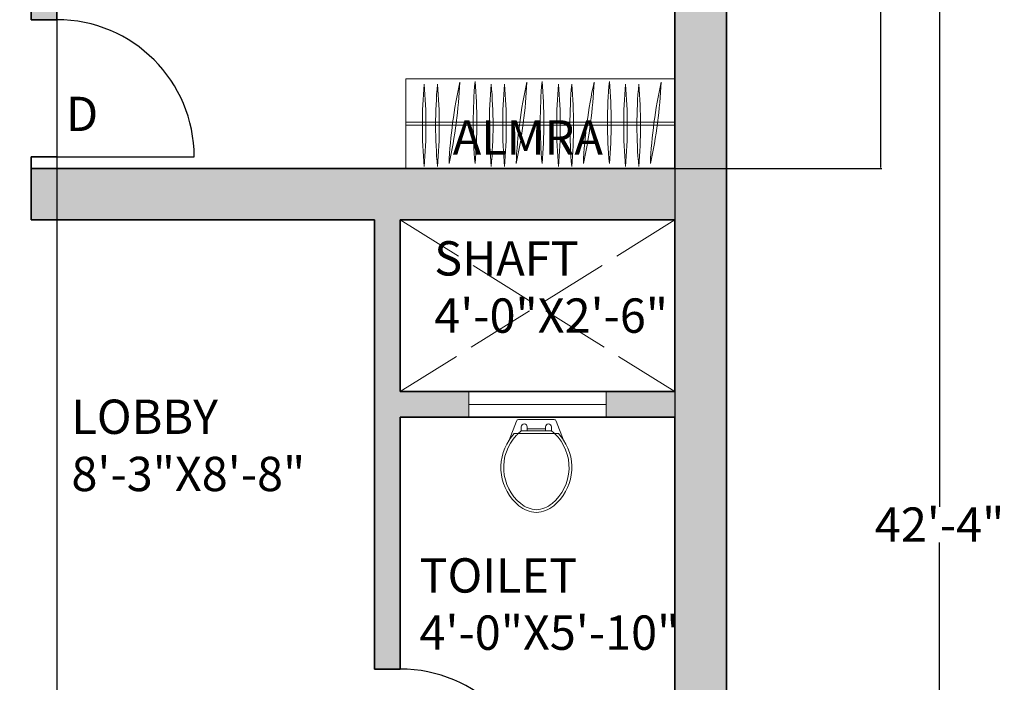
# Model space of a CAD drawing. Units: inches. Extents: x -5 to 330, y -522 to 40.
# Tile 22 of 23: x 158 to 330, y -269 to -153. Entities that reach past the tile are written whole.
import ezdxf

# ---------------------------------------------------------------- set-up
doc = ezdxf.new("R2010")
doc.units = ezdxf.units.IN
doc.header["$MEASUREMENT"] = 0
doc.linetypes.add('ACAD_ISO02W100', pattern=[15, 12, -3])
for name, color, linetype, lineweight in [('A-ANNO-DIMS', 2, 'Continuous', 18), ('A-ANNO-TEXT', 7, 'Continuous', 18), ('A-AREA-IDEN', 7, 'Continuous', 25), ('A-DOOR', 4, 'Continuous', 25), ('A-FLOR-OPEN', 8, 'ACAD_ISO02W100', 18), ('A-FURN', 8, 'Continuous', 18), ('A-GLAZ', 4, 'Continuous', 18), ('A-WALL', 7, 'Continuous', 35), ('WC-Detail_dwgmodels.com', 251, 'Continuous', 13), ('WC-Outline_dwgmodels.com', 250, 'Continuous', 18)]:
    doc.layers.add(name, color=color, linetype=linetype, lineweight=lineweight)
doc.layers.add('A-WALL-PATT', color=18, linetype='Continuous', lineweight=13, true_color=0x000000)
doc.styles.get("Standard").update_dxf_attribs({"font": 'arial.ttf'})
doc.dimstyles.get("Standard").update_dxf_attribs({"dimtxt": 0.18, "dimasz": 0.18, "dimexe": 0.18, "dimexo": 0.0625, "dimgap": 0.09, "dimtad": 0, "dimtih": 1, "dimtoh": 1, "dimdec": 0, "dimzin": 0, "dimdsep": 46, "dimlunit": 3, "dimtxsty": 'Standard', "dimcen": 0.09, "dimadec": 0, "dimazin": 0, "dimtfac": 1, "dimtdec": 0, "dimtofl": 0, "dimtmove": 0, "dimatfit": 3, "dimfxl": 1, "dimtolj": 1, "dimtzin": 0, "dimarcsym": 0})

# ---------------------------------------------------------------- blocks, each defined once
blk = doc.blocks.new('*D6')
at = {"layer": 'A-ANNO-DIMS', "color": 0, "lineweight": -2, "transparency": 16777216}
for p, q in [((281.07, 12.36), (318.43, 12.36)), ((318.25, 12.18), (318.25, -238.29)), ((318.25, -494.96), (318.25, -244.5)), ((281.07, -495.14), (318.43, -495.14))]:
    blk.add_line(p, q, dxfattribs=at)
at = {"layer": 'A-ANNO-DIMS', "color": 0, "transparency": 16777216}
for points in [[(318.22, 12.18), (318.28, 12.18), (318.25, 12.36)], [(318.22, -494.96), (318.28, -494.96), (318.25, -495.14)]]:
    blk.add_solid(points, dxfattribs=at)
at = {"layer": 'Defpoints', "color": 0, "transparency": 16777216}
for p in [(281.01, 12.36), (281.01, -495.14), (318.25, -495.14)]:
    blk.add_point(p, dxfattribs=at)
at = {"layer": 'A-ANNO-DIMS', "color": 0, "transparency": 16777216, "insert": (318.25, -241.39), "char_height": 6, "attachment_point": 5}
blk.add_mtext('\\A1;42\'-4"', dxfattribs=at)
blk = doc.blocks.new('DOOR-24IN-SWING')
blk.add_line((24, 0), (24, 24))
blk.add_arc((24, 0), 24, 90, 180)
blk = doc.blocks.new('WARDROBE-47IN')
for p, q in [((47.01, 15.67), (0, 15.67)), ((0, 15.67), (0, 0)), ((47.01, 15.67), (47.01, 0)), ((47.01, 8.1), (0, 8.1)), ((47.01, 7.57), (0, 7.57)), ((47.01, 0), (0, 0))]:
    blk.add_line(p, q)
for centre, start, end in [((85.32, 7.52), 175.0028, 184.9972), ((-78.95, 7.52), 355.0028, 4.9972), ((87.64, 7.52), 175.0028, 184.9972), ((-76.62, 7.52), 355.0028, 4.9972), ((-72.96, 18.68), 347.508, 357.5023), ((89.91, -2.75), 167.508, 177.5023), ((94.21, 8.03), 175.0028, 184.9972), ((-70.06, 8.03), 355.0028, 4.9972), ((97.03, 7.52), 175.0028, 184.9972), ((-67.23, 7.52), 355.0028, 4.9972), ((99.36, 7.52), 175.0028, 184.9972), ((-64.91, 7.52), 355.0028, 4.9972), ((-61.24, 18.68), 347.508, 357.5023), ((101.62, -2.75), 167.508, 177.5023), ((105.92, 8.03), 175.0028, 184.9972), ((-58.34, 8.03), 355.0028, 4.9972), ((108.79, 7.52), 175.0028, 184.9972), ((-55.48, 7.52), 355.0028, 4.9972), ((111.11, 7.52), 175.0028, 184.9972), ((-53.16, 7.52), 355.0028, 4.9972), ((113.38, -2.75), 167.508, 177.5023), ((-49.49, 18.68), 347.508, 357.5023), ((117.68, 8.03), 175.0028, 184.9972), ((-46.59, 8.03), 355.0028, 4.9972), ((120.5, 7.52), 175.0028, 184.9972), ((-43.77, 7.52), 355.0028, 4.9972), ((122.82, 7.52), 175.0028, 184.9972), ((-41.45, 7.52), 355.0028, 4.9972), ((125.09, -2.75), 167.508, 177.5023), ((-37.78, 18.68), 347.508, 357.5023)]:
    blk.add_arc(centre, 82.45, start, end)
blk = doc.blocks.new('*D37')
at = {"layer": 'A-ANNO-DIMS', "color": 0, "lineweight": -2, "transparency": 16777216}
for p, q in [((164.01, -53.21), (164.01, -522.31)), ((272.01, -53.21), (272.01, -522.31)), ((164.19, -522.13), (217.68, -522.13)), ((271.83, -522.13), (218.34, -522.13))]:
    blk.add_line(p, q, dxfattribs=at)
at = {"layer": 'A-ANNO-DIMS', "color": 0, "transparency": 16777216}
for points in [[(164.19, -522.1), (164.19, -522.16), (164.01, -522.13)], [(271.83, -522.1), (271.83, -522.16), (272.01, -522.13)]]:
    blk.add_solid(points, dxfattribs=at)
at = {"layer": 'Defpoints', "color": 0, "transparency": 16777216}
for p in [(164.01, -53.14), (272.01, -53.14), (272.01, -522.13)]:
    blk.add_point(p, dxfattribs=at)
at = {"layer": 'A-ANNO-DIMS', "color": 0, "transparency": 16777216, "insert": (218.01, -522.13), "char_height": 0.18, "attachment_point": 5}
blk.add_mtext('\\A1;9\'-0"', dxfattribs=at)
blk = doc.blocks.new('*D38')
at = {"layer": 'A-ANNO-DIMS', "color": 0, "lineweight": -2, "transparency": 16777216}
for p, q in [((272.07, -53.14), (308.17, -53.14)), ((307.99, -53.32), (307.99, -115.96)), ((307.99, -178.96), (307.99, -116.33)), ((272.07, -179.14), (308.17, -179.14))]:
    blk.add_line(p, q, dxfattribs=at)
at = {"layer": 'A-ANNO-DIMS', "color": 0, "transparency": 16777216}
for points in [[(307.96, -53.32), (308.02, -53.32), (307.99, -53.14)], [(307.96, -178.96), (308.02, -178.96), (307.99, -179.14)]]:
    blk.add_solid(points, dxfattribs=at)
at = {"layer": 'Defpoints', "color": 0, "transparency": 16777216}
for p in [(272.01, -53.14), (272.01, -179.14), (307.99, -179.14)]:
    blk.add_point(p, dxfattribs=at)
at = {"layer": 'A-ANNO-DIMS', "color": 0, "transparency": 16777216, "insert": (307.99, -116.14), "char_height": 0.18, "attachment_point": 5}
blk.add_mtext('\\A1;10\'-6"', dxfattribs=at)

msp = doc.modelspace()

# ---------------------------------------------------------------- hatches: boundary and pattern name
at = {"layer": 'A-WALL-PATT'}
h = msp.add_hatch(color=256, dxfattribs=at)
h.dxf.hatch_style = 1
h.paths.add_polyline_path([(164.01, -44.15), (159.51, -44.15), (159.51, -153.14), (164.01, -153.14)], flags=17)
h.paths.add_polyline_path([(224.01, -188.14), (272.01, -188.14), (272.01, -218.14), (260.01, -218.14), (260.01, -222.64), (272.01, -222.64), (272.01, -292.64), (159.01, -292.64), (159.01, -297.14), (272.01, -297.14), (272.01, -417.14), (245.51, -417.14), (245.51, -426.14), (272.01, -426.14), (272.01, -495.14), (281.01, -495.14), (281.01, 12.36), (23.51, 12.36), (23.51, -426.14), (62.92, -426.14), (62.92, -417.14), (32.51, -417.14), (32.51, -297.14), (48.13, -297.14), (48.13, -292.64), (32.51, -292.64), (32.51, -140.64), (133.51, -140.64), (133.51, -131.64), (32.51, -131.64), (32.51, 3.36), (159.51, 3.36), (164.01, 3.36), (220.01, 3.36), (224.51, 3.36), (272.01, 3.36), (272.01, -179.14), (159.51, -179.14), (159.51, -188.14), (219.51, -188.14), (219.51, -266.64), (224.01, -266.64), (224.01, -222.64), (236.01, -222.64), (236.01, -218.14), (224.01, -218.14)])
h.paths.add_polyline_path([(133.01, -292.64), (128.51, -292.64), (128.51, -297.14), (128.51, -417.14), (122.92, -417.14), (122.92, -426.14), (133.01, -426.14)], flags=17)
h.paths.add_polyline_path([(185.51, -417.14), (159.01, -417.14), (159.01, -426.14), (185.51, -426.14)], flags=17)
h.paths.add_polyline_path([(133.51, -140.64), (129.01, -140.64), (129.01, -246.64), (133.51, -246.64)], flags=17)
h.paths.add_polyline_path([(246.01, -48.64), (224.51, -48.64), (224.51, -27.63), (220.01, -27.63), (220.01, -48.64), (198.6, -48.64), (198.6, -53.14), (246.01, -53.14)], flags=17)

# ---------------------------------------------------------------- linework, layer by layer
at = {"layer": 'A-FLOR-OPEN'}
for p, q in [((224.01, -188.14), (272.01, -218.14)), ((272.01, -188.14), (224.01, -218.14))]:
    msp.add_line(p, q, dxfattribs=at)
at = {"layer": 'A-GLAZ'}
for p, q in [((236.01, -218.14), (260.01, -218.14)), ((236.01, -222.64), (236.01, -218.14)), ((260.01, -218.14), (260.01, -222.64)), ((236.01, -220.39), (260.01, -220.39)), ((260.01, -222.64), (236.01, -222.64))]:
    msp.add_line(p, q, dxfattribs=at)
at = {"layer": 'A-WALL'}
for p, q in [((281.01, 12.36), (281.01, -495.14)), ((159.51, 3.36), (159.51, -153.14)), ((164.01, 3.36), (164.01, -153.14)), ((272.01, 3.36), (272.01, -179.14)), ((159.51, -153.14), (164.01, -153.14)), ((159.51, -177.14), (164.01, -177.14)), ((159.51, -177.14), (159.51, -188.14)), ((159.51, -179.14), (272.01, -179.14)), ((159.51, -188.14), (219.51, -188.14)), ((219.51, -188.14), (219.51, -266.64)), ((224.01, -188.14), (224.01, -218.14)), ((224.01, -188.14), (272.01, -188.14)), ((272.01, -188.14), (272.01, -218.14)), ((224.01, -218.14), (272.01, -218.14)), ((224.01, -222.64), (272.01, -222.64)), ((224.01, -222.64), (224.01, -266.64)), ((272.01, -222.64), (272.01, -292.64)), ((224.01, -266.64), (219.51, -266.64))]:
    msp.add_line(p, q, dxfattribs=at)
at = {"layer": 'WC-Detail_dwgmodels.com'}
for p, q in [((243.92, -225.49), (244.6, -225.49)), ((250.98, -225.49), (251.66, -225.49))]:
    msp.add_line(p, q, dxfattribs=at)
for points in [[(245.16, -225, 0.022712), (244.6, -225.49, 0.162618)], [(245.16, -225), (245.16, -224.32, -1), (246.19, -224.32), (246.19, -224.67)], [(247.79, -225), (245.16, -225, 0.022712)], [(247.79, -225), (250.42, -225, -0.476108)], [(250.42, -225), (250.42, -224.32, 1), (249.39, -224.32), (249.39, -224.67)], [(250.42, -225, -0.022712), (250.98, -225.49, -0.162618)], [(243.92, -225.49, 0.040937), (243.04, -226.61, 0.163732)], [(251.66, -225.49, -0.040937), (252.54, -226.61, -0.163732)]]:
    msp.add_lwpolyline(points, format="xyb", dxfattribs=at)
for points in [[(249.39, -224.67), (246.19, -224.67)], [(246.19, -224.67), (246.19, -225)], [(249.39, -224.67), (249.39, -225)]]:
    msp.add_lwpolyline(points, dxfattribs=at)
at = {"layer": 'WC-Outline_dwgmodels.com'}
for p in [(244.6, -225.49), (250.98, -225.49)]:
    msp.add_line(p, (247.79, -225.49), dxfattribs=at)
for points in [[(247.79, -223.03), (244.69, -223.03, 0.31031), (244.31, -223.3), (243.04, -226.61, 0.209071)], [(247.79, -223.03), (250.89, -223.03, -0.31031), (251.27, -223.3), (252.54, -226.61, -0.209071)], [(243.04, -226.61, 0.383919), (244.74, -238.09, 0.163732), (247.79, -239.26, 0.359733)], [(244.27, -225.82, 0.431639), (245.05, -237.72, 0.162618), (247.79, -238.78, 0.470877)], [(244.6, -225.49, 0.014165), (244.27, -225.82, 0.162618)], [(250.98, -225.49, -0.448546), (250.53, -237.72, -0.162618), (247.79, -238.78, -0.470877)], [(252.54, -226.61, -0.383919), (250.84, -238.09, -0.163732), (247.79, -239.26, -0.359733)]]:
    msp.add_lwpolyline(points, format="xyb", dxfattribs=at)

# ---------------------------------------------------------------- block references
at = {"layer": 'A-DOOR'}
for p, rotation in [((164.01, -153.14), 270), ((224.01, -266.64), 269.9999999999999)]:
    msp.add_blockref('DOOR-24IN-SWING', p, dxfattribs=dict(at, rotation=rotation))
at = {"layer": 'A-FURN'}
msp.add_blockref('WARDROBE-47IN', (225, -179.14), dxfattribs=at)

# ---------------------------------------------------------------- texts
at = {"layer": 'A-ANNO-TEXT', "insert": (165.59, -166.61), "char_height": 6, "attachment_point": 1}
msp.add_mtext('D', dxfattribs=at)
at = {"layer": 'A-ANNO-TEXT', "insert": (233.18, -170.72), "char_height": 6, "attachment_point": 1}
msp.add_mtext_dynamic_manual_height_columns('ALMRA', width=37.1962, gutter_width=1, heights=[0], dxfattribs=at)
at = {"layer": 'A-AREA-IDEN', "char_height": 6, "attachment_point": 1}
for s, insert in [('SHAFT\\P4\'-0"X2\'-6"', (229.95, -191.86)), ('LOBBY\\P8\'-3"X8\'-8"', (166.55, -219.54)), ('TOILET\\P4\'-0"X5\'-10"', (227.37, -247.27))]:
    msp.add_mtext(s, dxfattribs=dict(at, insert=insert))

# ---------------------------------------------------------------- dimensions: what is measured, and where the dimension line sits
at = {"layer": 'A-ANNO-DIMS'}
for base, p1, p2, override, picture, middle in [((318.24603734, -495.14358203), (281.00988858, 12.35641797), (281.00988858, -495.14358203), {"dimtxt": 6, "dimclrd": 0, "dimclre": 0, "dimclrt": 0}, '*D6', (318.24603734, -241.39358203)), ((307.99, -179.14), (272.01, -53.14), (272.01, -179.14), {"dimdec": 1, "dimlfac": 1, "dimrnd": 0, "dimzin": 1, "dimdsep": 46, "dimlunit": 4, "dimfrac": 2}, '*D38', (307.99, -116.14))]:
    dim = msp.add_linear_dim(base=base, p1=p1, p2=p2, angle=90, dimstyle='Standard', override=override, dxfattribs=at)
    dim.commit()
    dim.dimension.update_dxf_attribs({"geometry": picture, "text_midpoint": middle})
dim = msp.add_linear_dim(base=(272.01, -522.13), p1=(164.01, -53.14), p2=(272.01, -53.14), dimstyle='Standard', override={"dimdec": 1, "dimlfac": 1, "dimrnd": 0, "dimzin": 1, "dimdsep": 46, "dimlunit": 4, "dimfrac": 2}, dxfattribs=at)
dim.commit()
dim.dimension.update_dxf_attribs({"geometry": '*D37', "text_midpoint": (218.01, -522.13)})

doc.saveas('drawing.dxf')
